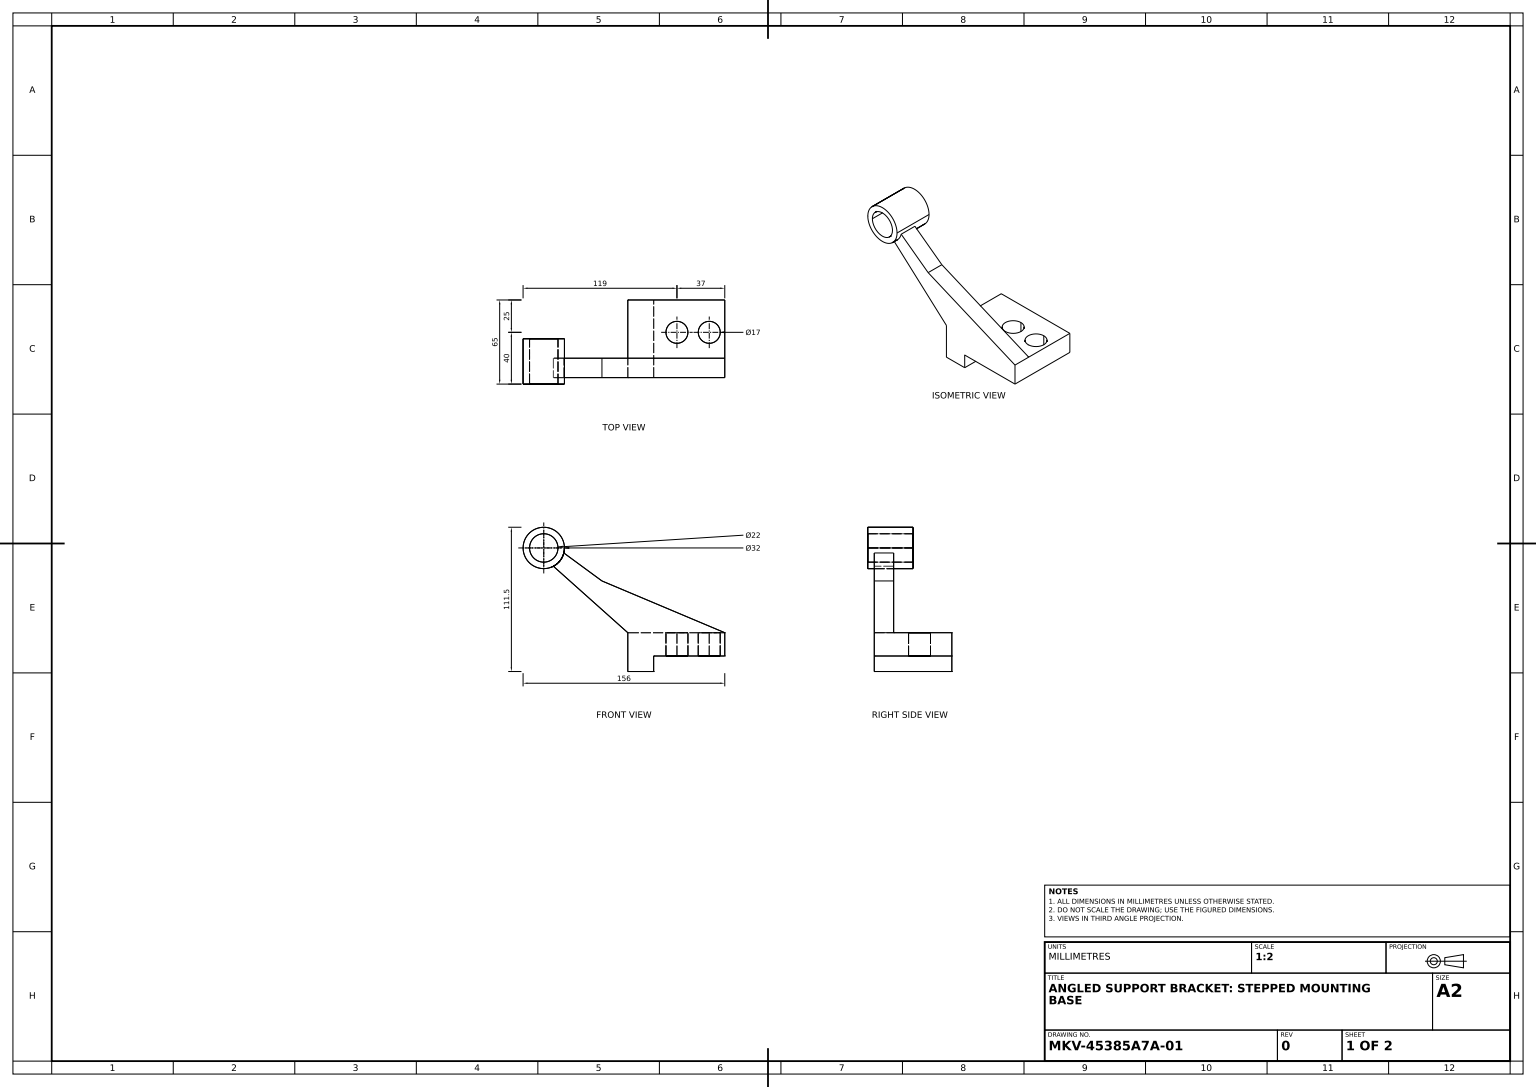
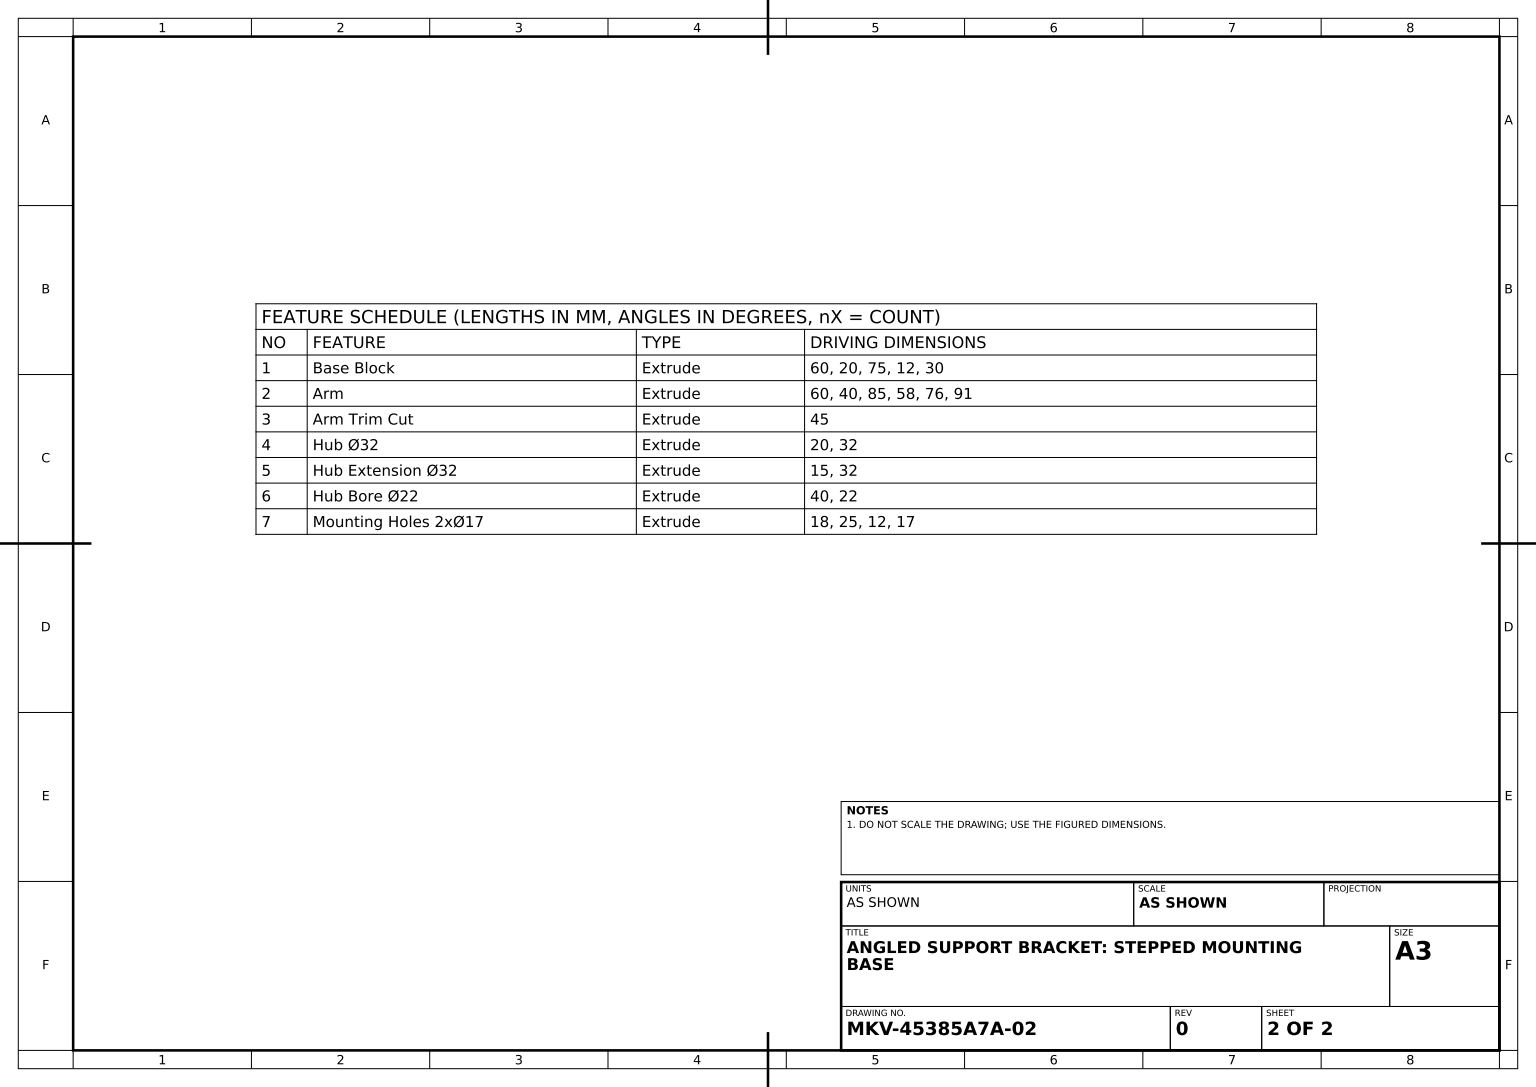
from build123d import *

# Parameters (mm, degrees)
BASE_BLOCK_DEPTH           = 60
ARM_DEPTH                  = 60
ARM_TRIM_CUT_DEPTH         = 45
HUB_SKETCH_32_R            = 16
HUB_32_DEPTH               = 20
HUB_START                  = 15
HUB_EXTENSION_SKETCH_32_R  = 16
HUB_EXTENSION_32_DEPTH     = 15
BORE_SKETCH_22_R           = 11
HUB_BORE_22_DEPTH          = 40
MOUNTING_HOLES_SKETCH_R    = 8.5
MOUNTING_HOLES_2X_17_DEPTH = 18


with BuildPart() as part:
    # Base Profile Sketch → Base Block (new body)
    with BuildSketch(Plane.XY):
        Polygon((0, 0), (-75, 0), (-75, -30), (-55, -30), (-55, -18), (0, -18), align=None)
    extrude(amount=BASE_BLOCK_DEPTH)

    # Arm Profile Sketch → Arm (add)
    with BuildSketch(Plane(origin=(0, 0, 0), x_dir=(-1, 0, 0), z_dir=(0, 0, -1))):
        Polygon((0, 0), (75, 0), (140, 58), (140, 73), (95, 40), align=None)
    extrude(amount=-ARM_DEPTH)

    # Arm Trim Sketch → Arm Trim Cut (cut)
    with BuildSketch(Plane(origin=(0, 0, 0), x_dir=(-1, 0, 0), z_dir=(0, 0, -1))):
        Polygon((0, 0), (95, 40), (140, 73), (140, 58), (75, 0), align=None)
    extrude(amount=-ARM_TRIM_CUT_DEPTH, mode=Mode.SUBTRACT)

    # Hub Sketch Ø32 → Hub Ø32 (add)
    with BuildSketch(Plane(origin=(0, 0, 45), x_dir=(-1, 0, 0), z_dir=(0, 0, -1))):
        with Locations((140, 65.5)):
            Circle(HUB_SKETCH_32_R)
    extrude(amount=-HUB_32_DEPTH)

    # Hub Extension Sketch Ø32 → Hub Extension Ø32 (add)
    with BuildSketch(Plane(origin=(0, 0, 45), x_dir=(-1, 0, 0), z_dir=(0, 0, -1)).offset(HUB_START)):
        with Locations((140, 65.5)):
            Circle(HUB_EXTENSION_SKETCH_32_R)
    extrude(amount=-HUB_EXTENSION_32_DEPTH)

    # Bore Sketch Ø22 → Hub Bore Ø22 (cut)
    with BuildSketch(Plane(origin=(0, 0, 30), x_dir=(-1, 0, 0), z_dir=(0, 0, -1))):
        with Locations((140, 65.5)):
            Circle(BORE_SKETCH_22_R)
    extrude(amount=-HUB_BORE_22_DEPTH, mode=Mode.SUBTRACT)

    # Mounting Holes Sketch → Mounting Holes 2xØ17 (cut)
    with BuildSketch(Plane(origin=(0, 0, 0), x_dir=(1, 0, 0), z_dir=(0, 1, 0))):
        with Locations(Location((-12, -25, 0), (0, 0, 270))):
            Circle(MOUNTING_HOLES_SKETCH_R)
        with Locations(Location((-37, -25, 0), (0, 0, 270))):
            Circle(MOUNTING_HOLES_SKETCH_R)
    extrude(amount=-MOUNTING_HOLES_2X_17_DEPTH, mode=Mode.SUBTRACT)


solid = part.part
